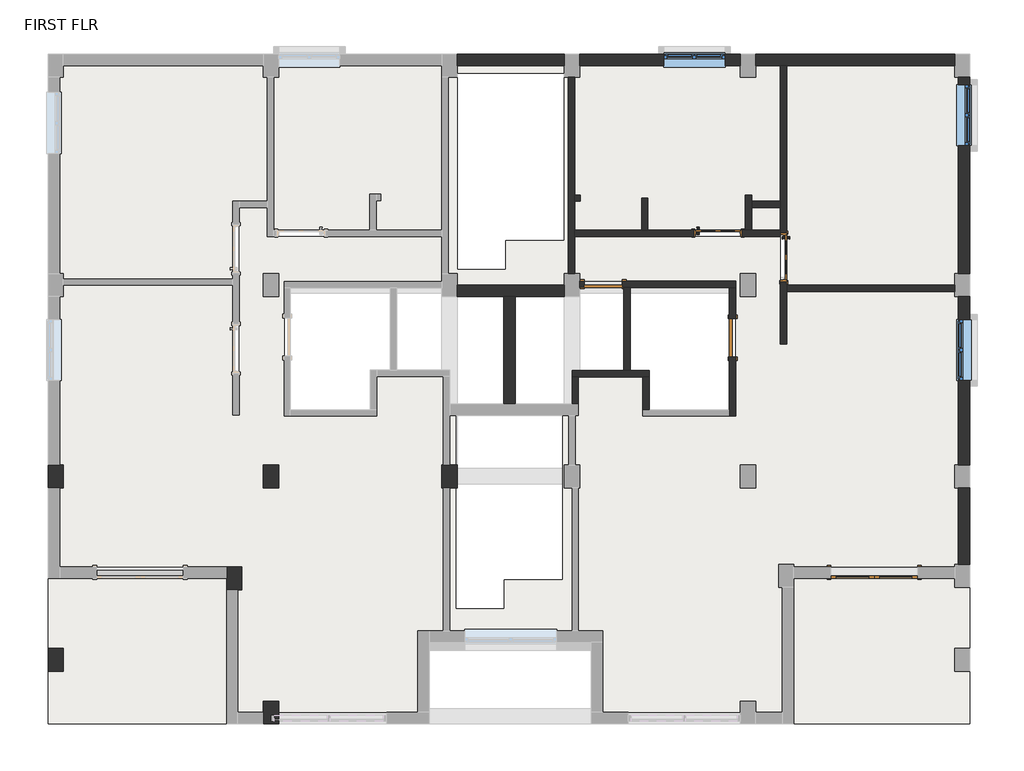
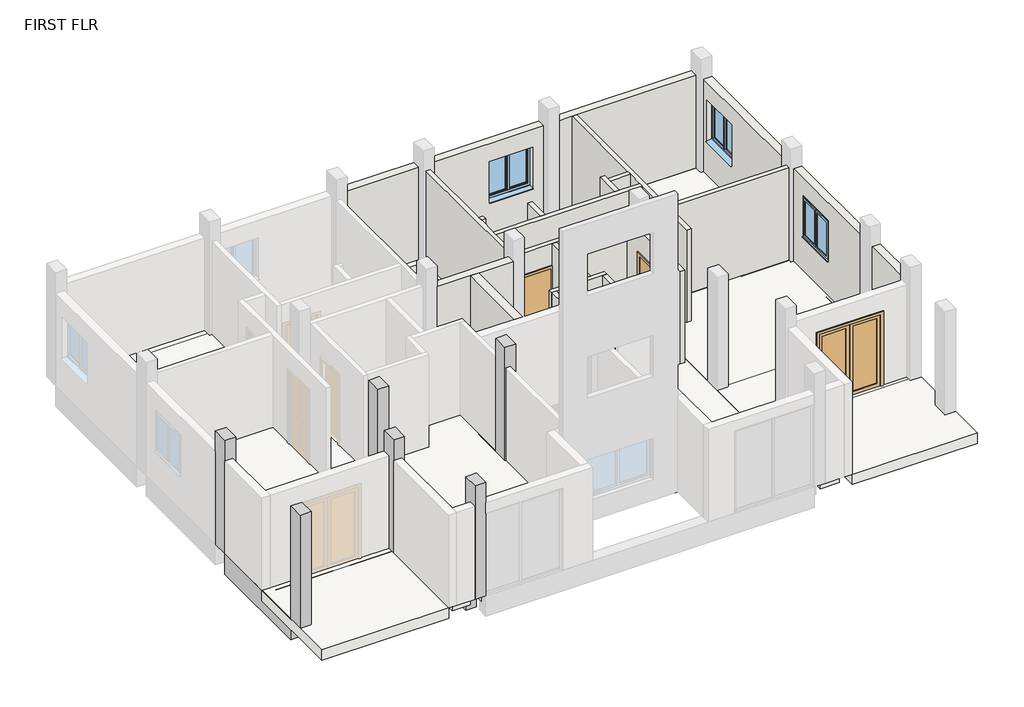
# One storey, part 2 of 3: 22 walls, 7 slabs, 6 beams, 6 columns, 5 doors, 3 windows.
"""IFC4 building model written with IfcOpenShell, lengths in millimetres."""

from ifc_helpers import new_model, si_unit, frame, origin, place, context, project, spatial, polyline, outline, extrude, faceted_brep, transform, mapped, element, save
from components import door_e52a3823, door_68a706ac, door_1fe7f57d, w2_0001_windows_4_x_4_9dec5fc7

model = new_model("IFC4")

# Units and contexts
model_context = context("Model", 3, world=origin())
ifc_project = project(units=[si_unit("LENGTHUNIT", "METRE", prefix="MILLI")], contexts=[model_context])

# Site, building, storey
site = spatial("IfcSite", under=ifc_project)
building = spatial("IfcBuilding", under=site)
storey = spatial("IfcBuildingStorey", under=building, Name="FIRST FLR", Elevation=3352.8)

# Beams
placement = place(None, origin())
element("IfcBeam", 1, ObjectType="Concrete-Rectangular Beam : 12 x 24", at=placement, inside=storey, context=model_context, shape_type="Brep", body=[
    faceted_brep([(-9144.7786397, -13068.2620333, 3352.8), (-8839.9786397, -13068.2620333, 3352.8), (-8839.9786397, -11823.6620333, 3352.8), (-8839.9786397, -11518.8620333, 3352.8), (-8839.9786397, -9867.8620333, 3352.8), (-9144.7786397, -9867.8620333, 3352.8), (-9144.7786397, -13068.2620333, 2743.2), (-9144.7786397, -9867.8620333, 2743.2), (-8839.9786397, -13068.2620333, 2743.2), (-8839.9786397, -9867.8620333, 2743.2), (-8839.9786397, -11518.8620333, 2743.2), (-8839.9786397, -11823.6620333, 2743.2)], [[[0, 1, 2, 3, 4, 5]], [[6, 0, 5, 7]], [[8, 6, 7, 9, 10, 11]], [[1, 8, 11, 10, 9, 4, 3, 2]], [[4, 9, 7, 5]], [[1, 0, 6, 8]]]),
])
element("IfcBeam", 2, ObjectType="Concrete-Rectangular Beam : 12 x 24", at=placement, inside=storey, context=model_context, shape_type="SweptSolid", body=[
    extrude(outline(polyline([(-4852.9175798, -9486.8620333), (-4852.9175798, -9791.6620333), (-8839.9786397, -9791.6620333), (-8839.9786397, -9486.8620333), (-4852.9175798, -9486.8620333)])), frame((0.0, 0.0, 2743.2), z_axis=(0.0, 0.0, 1.0), x_axis=(1.0, 0.0, 0.0)), (0.0, 0.0, 1.0), 609.6),
])
element("IfcBeam", 3, ObjectType="Concrete-Rectangular Beam : 12 x 24", at=placement, inside=storey, context=model_context, shape_type="SweptSolid", body=[
    extrude(outline(polyline([(-1296.9175798, -9486.8620333), (-1296.9175798, -9791.6620333), (-4548.1175798, -9791.6620333), (-4548.1175798, -9486.8620333), (-1296.9175798, -9486.8620333)])), frame((0.0, 0.0, 2743.2), z_axis=(0.0, 0.0, 1.0), x_axis=(1.0, 0.0, 0.0)), (0.0, 0.0, 1.0), 609.6),
])
element("IfcBeam", 4, ObjectType="Concrete-Rectangular Beam : 12 x 24", at=placement, inside=storey, context=model_context, shape_type="Brep", body=[
    faceted_brep([(-4852.9175798, -14119.6402089, 3352.8), (-4548.1175798, -14119.6402089, 3352.8), (-4548.1175798, -9867.8620333, 3352.8), (-4852.9175798, -9867.8620333, 3352.8), (-4852.9175798, -11518.8620333, 3352.8), (-4852.9175798, -11823.6620333, 3352.8), (-4852.9175798, -14119.6402089, 2743.2), (-4852.9175798, -9867.8620333, 2743.2), (-4852.9175798, -11518.8620333, 2743.2), (-4852.9175798, -11823.6620333, 2743.2), (-4548.1175798, -14119.6402089, 2743.2), (-4548.1175798, -9867.8620333, 2743.2)], [[[0, 1, 2, 3, 4, 5]], [[6, 0, 5, 4, 3, 7, 8, 9]], [[10, 6, 9, 8, 7, 11]], [[1, 10, 11, 2]], [[2, 11, 7, 3]], [[1, 0, 6, 10]]]),
])
element("IfcBeam", 5, ObjectType="Concrete-Rectangular Beam : 12 x 24", at=placement, inside=storey, context=model_context, shape_type="SweptSolid", body=[
    extrude(outline(polyline([(-5284.7175798, -11823.6620333), (-5284.7175798, -11518.8620333), (-4852.9175798, -11518.8620333), (-4852.9175798, -11823.6620333), (-5284.7175798, -11823.6620333)])), frame((0.0, 0.0, 2743.2), z_axis=(0.0, 0.0, 1.0), x_axis=(1.0, 0.0, 0.0)), (0.0, 0.0, 1.0), 609.6),
])
element("IfcBeam", 6, ObjectType="Concrete-Rectangular Beam : 12 x 24", at=placement, inside=storey, context=model_context, shape_type="SweptSolid", body=[
    extrude(outline(polyline([(-5589.5175798, -11518.8620333), (-5589.5175798, -11823.6620333), (-8839.9786397, -11823.6620333), (-8839.9786397, -11518.8620333), (-5589.5175798, -11518.8620333)])), frame((0.0, 0.0, 2743.2), z_axis=(0.0, 0.0, 1.0), x_axis=(1.0, 0.0, 0.0)), (0.0, 0.0, 1.0), 609.6),
])

# Columns
element("IfcColumn", 7, ObjectType="Concrete-Rectangular-Column : 1'6\" X 1' COLUMN", at=placement, inside=storey, context=model_context, shape_type="Brep", body=[
    faceted_brep([(-8839.9786397, -9410.6620333, 3352.8), (-8839.9786397, -9867.8620333, 3352.8), (-9144.7786397, -9867.8620333, 3352.8), (-9144.7786397, -9410.6620333, 3352.8), (-8839.9786397, -9410.6620333, 6705.6), (-8839.9786397, -9486.8620333, 6705.6), (-8839.9786397, -9791.6620333, 6705.6), (-8839.9786397, -9867.8620333, 6705.6), (-8839.9786397, -9867.8620333, 6096.0), (-8839.9786397, -9867.8620333, 5791.2), (-8839.9786397, -9410.6620333, 5791.2), (-8839.9786397, -9410.6620333, 6096.0), (-9144.7786397, -9867.8620333, 6705.6), (-9144.7786397, -9867.8620333, 6096.0), (-9144.7786397, -9867.8620333, 5791.2), (-9144.7786397, -9410.6620333, 6705.6), (-9144.7786397, -9410.6620333, 6096.0), (-9144.7786397, -9410.6620333, 5791.2)], [[[0, 1, 2, 3]], [[4, 5, 6, 7, 8, 9, 1, 0, 10, 11]], [[7, 12, 13, 14, 2, 1, 9, 8]], [[12, 15, 16, 17, 3, 2, 14, 13]], [[15, 4, 11, 10, 0, 3, 17, 16]], [[4, 15, 12, 7, 6, 5]]]),
])
element("IfcColumn", 8, ObjectType="Concrete-Rectangular-Column : 1'6\" X 1' COLUMN", at=placement, inside=storey, context=model_context, shape_type="Brep", body=[
    faceted_brep([(-4548.1175798, -9410.6620333, 3352.8), (-4548.1175798, -9867.8620333, 3352.8), (-4852.9175798, -9867.8620333, 3352.8), (-4852.9175798, -9410.6620333, 3352.8), (-4548.1175798, -9410.6620333, 6705.6), (-4548.1175798, -9486.8620333, 6705.6), (-4548.1175798, -9791.6620333, 6705.6), (-4548.1175798, -9867.8620333, 6705.6), (-4548.1175798, -9867.8620333, 6096.0), (-4548.1175798, -9867.8620333, 5791.2), (-4548.1175798, -9410.6620333, 5791.2), (-4548.1175798, -9410.6620333, 6096.0), (-4852.9175798, -9867.8620333, 6705.6), (-4852.9175798, -9867.8620333, 6096.0), (-4852.9175798, -9867.8620333, 5791.2), (-4852.9175798, -9791.6620333, 6705.6), (-4852.9175798, -9486.8620333, 6705.6), (-4852.9175798, -9410.6620333, 6705.6), (-4852.9175798, -9410.6620333, 6096.0), (-4852.9175798, -9410.6620333, 5791.2)], [[[0, 1, 2, 3]], [[4, 5, 6, 7, 8, 9, 1, 0, 10, 11]], [[7, 12, 13, 14, 2, 1, 9, 8]], [[12, 15, 16, 17, 18, 19, 3, 2, 14, 13]], [[17, 4, 11, 10, 0, 3, 19, 18]], [[4, 17, 16, 15, 12, 7, 6, 5]]]),
])
element("IfcColumn", 9, ObjectType="Concrete-Rectangular-Column : 1'6\" X 1' COLUMN", at=placement, inside=storey, context=model_context, shape_type="Brep", body=[
    faceted_brep([(-992.1175798, -9410.6620333, 3352.8), (-992.1175798, -9867.8620333, 3352.8), (-1296.9175798, -9867.8620333, 3352.8), (-1296.9175798, -9410.6620333, 3352.8), (-992.1175798, -9410.6620333, 6705.6), (-992.1175798, -9867.8620333, 6705.6), (-992.1175798, -9410.6620333, 5791.2), (-992.1175798, -9410.6620333, 6096.0), (-1296.9175798, -9867.8620333, 6705.6), (-1296.9175798, -9791.6620333, 6705.6), (-1296.9175798, -9486.8620333, 6705.6), (-1296.9175798, -9410.6620333, 6705.6), (-1296.9175798, -9410.6620333, 6096.0), (-1296.9175798, -9410.6620333, 5791.2)], [[[0, 1, 2, 3]], [[4, 5, 1, 0, 6, 7]], [[5, 8, 2, 1]], [[8, 9, 10, 11, 12, 13, 3, 2]], [[11, 4, 7, 6, 0, 3, 13, 12]], [[4, 11, 10, 9, 8, 5]]]),
])
element("IfcColumn", 10, ObjectType="Concrete-Rectangular-Column : 1'6\" X 1' COLUMN", at=placement, inside=storey, context=model_context, shape_type="Brep", body=[
    faceted_brep([(-4548.1175798, -14119.6402089, 3352.8), (-4548.1175798, -14576.8402089, 3352.8), (-4852.9175798, -14576.8402089, 3352.8), (-4852.9175798, -14119.6402089, 3352.8), (-4548.1175798, -14119.6402089, 6705.6), (-4548.1175798, -14576.8402089, 6705.6), (-4548.1175798, -14576.8402089, 6400.8), (-4548.1175798, -14576.8402089, 5791.2), (-4548.1175798, -14119.6402089, 5791.2), (-4548.1175798, -14119.6402089, 6096.0), (-4852.9175798, -14576.8402089, 6705.6), (-4852.9175798, -14119.6402089, 6705.6), (-4852.9175798, -14119.6402089, 6096.0), (-4852.9175798, -14119.6402089, 5791.2)], [[[0, 1, 2, 3]], [[4, 5, 6, 7, 1, 0, 8, 9]], [[5, 10, 2, 1, 7, 6]], [[10, 11, 12, 13, 3, 2]], [[11, 4, 9, 8, 0, 3, 13, 12]], [[4, 11, 10, 5]]]),
])
element("IfcColumn", 11, ObjectType="Concrete-Rectangular-Column : 1'6\" X 1' COLUMN", at=placement, inside=storey, context=model_context, shape_type="Brep", body=[
    faceted_brep([(-8839.9786397, -13068.2620333, 3352.8), (-8839.9786397, -13525.4620333, 3352.8), (-9144.7786397, -13525.4620333, 3352.8), (-9144.7786397, -13068.2620333, 3352.8), (-8839.9786397, -13068.2620333, 6705.6), (-8839.9786397, -13525.4620333, 6705.6), (-8839.9786397, -13068.2620333, 5791.2), (-8839.9786397, -13068.2620333, 6096.0), (-9144.7786397, -13525.4620333, 6705.6), (-9144.7786397, -13068.2620333, 6705.6), (-9144.7786397, -13068.2620333, 6096.0), (-9144.7786397, -13068.2620333, 5791.2)], [[[0, 1, 2, 3]], [[4, 5, 1, 0, 6, 7]], [[5, 8, 2, 1]], [[8, 9, 10, 11, 3, 2]], [[9, 4, 7, 6, 0, 3, 11, 10]], [[4, 9, 8, 5]]]),
])
element("IfcColumn", 12, ObjectType="Concrete-Rectangular-Column : 1'6\" X 1' COLUMN", at=placement, inside=storey, context=model_context, shape_type="SweptSolid", body=[
    extrude(outline(polyline([(-5284.7175798, -11442.6620333), (-5284.7175798, -11899.8620333), (-5589.5175798, -11899.8620333), (-5589.5175798, -11442.6620333), (-5284.7175798, -11442.6620333)])), frame((0.0, 0.0, 3352.8), z_axis=(0.0, 0.0, 1.0), x_axis=(1.0, 0.0, 0.0)), (0.0, 0.0, 1.0), 3352.8),
])

# Doors
door_shape = door_e52a3823(model_context)
element("IfcDoor", 13, ObjectType="Door-Double-Glass : 68\" x 84\"", at=placement, inside=storey, context=model_context, shape_type="MappedRepresentation", body=[
    mapped(door_shape, transform((7313.6824202, -11554.5807833, 3352.8), x_axis=(-1.0, 0.0, 0.0), y_axis=(0.0, -1.0, 0.0), z_axis=(0.0, 0.0, 1.0))),
])
door_2_shape = door_68a706ac(model_context)
element("IfcDoor", 14, ObjectType="Door-Interior-Single-4_Panel-Wood : 36\" x 84\"", at=placement, inside=storey, context=model_context, shape_type="MappedRepresentation", body=[
    mapped(door_2_shape, transform((4202.1824202, -4789.1311634, 3352.8), x_axis=(1.0, 0.0, 0.0), y_axis=(0.0, 1.0, 0.0), z_axis=(0.0, 0.0, 1.0))),
])
element("IfcDoor", 15, ObjectType="Door-Interior-Single-4_Panel-Wood : 36\" x 84\"", at=placement, inside=storey, context=model_context, shape_type="MappedRepresentation", body=[
    mapped(door_2_shape, transform((5513.4574202, -5274.9061634, 3352.8), x_axis=(0.0, -1.0, 0.0), y_axis=(1.0, 0.0, 0.0), z_axis=(0.0, 0.0, 1.0))),
])
door_3_shape = door_1fe7f57d(model_context)
element("IfcDoor", 16, ObjectType="Single-Flush : 30\" x 80\"", at=placement, inside=storey, context=model_context, shape_type="MappedRepresentation", body=[
    mapped(door_3_shape, transform((1916.1824202, -5810.8691591, 3352.8), x_axis=(-1.0, 0.0, 0.0), y_axis=(0.0, -1.0, 0.0), z_axis=(0.0, 0.0, 1.0))),
])
element("IfcDoor", 17, ObjectType="Single-Flush : 30\" x 80\"", at=placement, inside=storey, context=model_context, shape_type="MappedRepresentation", body=[
    mapped(door_3_shape, transform((4494.2824202, -6877.6691591, 3352.8), x_axis=(0.0, 1.0, 0.0), y_axis=(-1.0, 0.0, 0.0), z_axis=(0.0, 0.0, 1.0))),
])

# Slabs
element("IfcSlab", 18, ObjectType="flooring 1'", at=placement, inside=storey, context=model_context, shape_type="SweptSolid", body=[
    extrude(outline(polyline([(-8916.1786397, -11442.6620333), (-8916.1786397, -9867.8620333), (-8839.9786397, -9867.8620333), (-8839.9786397, -9410.6620333), (-8916.1786397, -9410.6620333), (-8916.1786397, -6057.8620333), (-8839.9786397, -6057.8620333), (-8839.9786397, -5829.2620333), (-5462.5175798, -5829.2620333), (-5462.5175798, -8420.0620333), (-5335.5175798, -8420.0620333), (-5335.5175798, -4280.3104011), (-4776.7175798, -4280.3104011), (-4776.7175798, -4855.8061634), (-1296.9175798, -4855.8061634), (-1296.9175798, -5600.6620333), (-1296.9175798, -5758.8942903), (-4442.5950401, -5758.8942903), (-4442.5950401, -8439.1120333), (-2601.0950401, -8439.1120333), (-2601.0950401, -7651.7120333), (-1271.5175798, -7651.7120333), (-1271.5175798, -9410.6620333), (-1296.9175798, -9410.6620333), (-1296.9175798, -9867.8620333), (-1271.5175798, -9867.8620333), (-1271.5175798, -12722.6402089), (-1779.5175798, -12722.6402089), (-1779.5175798, -14348.2402089), (-4548.1175798, -14348.2402089), (-4548.1175798, -14119.6402089), (-4852.9175798, -14119.6402089), (-4852.9175798, -14348.2402089), (-5360.9175798, -14348.2402089), (-5360.9175798, -11899.8620333), (-5284.7175798, -11899.8620333), (-5284.7175798, -11442.6620333), (-5589.5175798, -11442.6620333), (-8916.1786397, -11442.6620333)])), frame((0.0, 0.0, 3048.0), z_axis=(0.0, 0.0, 1.0), x_axis=(1.0, 0.0, 0.0)), (0.0, 0.0, 1.0), 304.8),
])
element("IfcSlab", 19, ObjectType="flooring 1'", at=placement, inside=storey, context=model_context, shape_type="SweptSolid", body=[
    extrude(outline(polyline([(5446.7824202, -4855.8061634), (5446.7824202, -6583.0061634), (5573.7824202, -6583.0061634), (5573.7824202, -5956.2620333), (8913.8824202, -5956.2620333), (8913.8824202, -6057.8620333), (8990.0824202, -6057.8620333), (8990.0824202, -9410.6620333), (8913.8824202, -9410.6620333), (8913.8824202, -9867.8620333), (8990.0824202, -9867.8620333), (8990.0824202, -11391.8620333), (8913.8824202, -11391.8620333), (8913.8824202, -11442.6620333), (5713.4824202, -11442.6620333), (5713.4824202, -11391.8620333), (5408.6824202, -11391.8620333), (5408.6824202, -11849.0620333), (5484.8824202, -11849.0620333), (5484.8824202, -14348.2402089), (4951.4824202, -14348.2402089), (4951.4824202, -14119.6402089), (4646.6824202, -14119.6402089), (4646.6824202, -14348.2402089), (1903.4824202, -14348.2402089), (1903.4824202, -12722.6402089), (1420.8824202, -12722.6402089), (1420.8824202, -9867.8620333), (1446.2824202, -9867.8620333), (1446.2824202, -9410.6620333), (1357.3824202, -9410.6620333), (1357.3824202, -8426.4120333), (1420.8824202, -8426.4120333), (1420.8824202, -7660.8890971), (2703.5824202, -7660.8890971), (2703.5824202, -8439.7691591), (4557.7824202, -8439.7691591), (4557.7824202, -5747.3691591), (1446.2824202, -5747.3691591), (1446.2824202, -5600.6620333), (1344.6824202, -5600.6620333), (1344.6824202, -4855.8061634), (5446.7824202, -4855.8061634)])), frame((0.0, 0.0, 3048.0), z_axis=(0.0, 0.0, 1.0), x_axis=(1.0, 0.0, 0.0)), (0.0, 0.0, 1.0), 304.8),
])
element("IfcSlab", 20, ObjectType="flooring 1'", at=placement, inside=storey, context=model_context, shape_type="SweptSolid", body=[
    extrude(outline(polyline([(-8839.9786397, -1680.8061634), (-8839.9786397, -1452.2061634), (-4852.9175798, -1452.2061634), (-4852.9175798, -1680.8061634), (-4776.7175798, -1680.8061634), (-4776.7175798, -4153.3104011), (-5462.5175798, -4153.3104011), (-5462.5175798, -5702.2620333), (-8839.9786397, -5702.2620333), (-8839.9786397, -5600.6620333), (-8916.1786397, -5600.6620333), (-8916.1786397, -1680.8061634), (-8839.9786397, -1680.8061634)])), frame((0.0, 0.0, 3048.0), z_axis=(0.0, 0.0, 1.0), x_axis=(1.0, 0.0, 0.0)), (0.0, 0.0, 1.0), 304.8),
    extrude(outline(polyline([(-2732.0175798, -4728.8061634), (-4649.7175798, -4728.8061634), (-4649.7175798, -1680.8061634), (-4548.1175798, -1680.8061634), (-4548.1175798, -1452.2061634), (-1296.9175798, -1452.2061634), (-1296.9175798, -4728.8061634), (-2605.0175798, -4728.8061634), (-2605.0175798, -4144.6061634), (-2516.1175798, -4144.6061634), (-2516.1175798, -4017.6061634), (-2732.0175798, -4017.6061634), (-2732.0175798, -4728.8061634)])), frame((0.0, 0.0, 3048.0), z_axis=(0.0, 0.0, 1.0), x_axis=(1.0, 0.0, 0.0)), (0.0, 0.0, 1.0), 304.8),
])
element("IfcSlab", 21, ObjectType="flooring 1'", at=placement, inside=storey, context=model_context, shape_type="SweptSolid", body=[
    extrude(outline(polyline([(4646.6824202, -1452.2061634), (4646.6824202, -1680.8061634), (4951.4824202, -1680.8061634), (4951.4824202, -1452.2061634), (5446.7824202, -1452.2061634), (5446.7824202, -4157.3061634), (4875.2824202, -4157.3061634), (4875.2824202, -4030.3061634), (4748.2824202, -4030.3061634), (4748.2824202, -4728.8061634), (2805.1824202, -4728.8061634), (2805.1824202, -4093.8061634), (2678.1824202, -4093.8061634), (2678.1824202, -4728.8061634), (1344.6824202, -4728.8061634), (1344.6824202, -4157.3061634), (1458.9824202, -4157.3061634), (1458.9824202, -4030.3061634), (1344.6824202, -4030.3061634), (1344.6824202, -1680.8061634), (1446.2824202, -1680.8061634), (1446.2824202, -1452.2061634), (4646.6824202, -1452.2061634)])), frame((0.0, 0.0, 3048.0), z_axis=(0.0, 0.0, 1.0), x_axis=(1.0, 0.0, 0.0)), (0.0, 0.0, 1.0), 304.8),
    extrude(outline(polyline([(5446.7824202, -4284.3061634), (5446.7824202, -4728.8061634), (4875.2824202, -4728.8061634), (4875.2824202, -4284.3061634), (5446.7824202, -4284.3061634)])), frame((0.0, 0.0, 3048.0), z_axis=(0.0, 0.0, 1.0), x_axis=(1.0, 0.0, 0.0)), (0.0, 0.0, 1.0), 304.8),
    extrude(outline(polyline([(8913.8824202, -5829.2620333), (5573.7824202, -5829.2620333), (5573.7824202, -1452.2061634), (8913.8824202, -1452.2061634), (8913.8824202, -1680.8061634), (8990.0824202, -1680.8061634), (8990.0824202, -5600.6620333), (8913.8824202, -5600.6620333), (8913.8824202, -5829.2620333)])), frame((0.0, 0.0, 3048.0), z_axis=(0.0, 0.0, 1.0), x_axis=(1.0, 0.0, 0.0)), (0.0, 0.0, 1.0), 304.8),
])
element("IfcSlab", 22, ObjectType="flooring 1'", at=placement, inside=storey, context=model_context, shape_type="SweptSolid", body=[
    extrude(outline(polyline([(1141.4824202, -1680.8061634), (1217.6824202, -1680.8061634), (1217.6824202, -5600.6620333), (1141.4824202, -5600.6620333), (1141.4824202, -5829.2620333), (-992.1175798, -5829.2620333), (-992.1175798, -5600.6620333), (-1169.9175798, -5600.6620333), (-1169.9175798, -1680.8061634), (-992.1175798, -1680.8061634), (-992.1175798, -5516.2061634), (-26.9175798, -5516.2061634), (-26.9175798, -4938.3561634), (1141.4824202, -4938.3561634), (1141.4824202, -1680.8061634)])), frame((0.0, 0.0, 3048.0), z_axis=(0.0, 0.0, 1.0), x_axis=(1.0, 0.0, 0.0)), (0.0, 0.0, 1.0), 304.8),
    extrude(outline(polyline([(-992.1175798, -1452.2061634), (1141.4824202, -1452.2061634), (1141.4824202, -1604.6061634), (-992.1175798, -1604.6061634), (-992.1175798, -1452.2061634)])), frame((0.0, 0.0, 3048.0), z_axis=(0.0, 0.0, 1.0), x_axis=(1.0, 0.0, 0.0)), (0.0, 0.0, 1.0), 304.8),
])
element("IfcSlab", 23, ObjectType="flooring 1'", at=placement, inside=storey, context=model_context, shape_type="SweptSolid", body=[
    extrude(outline(polyline([(1293.8824202, -12722.6402089), (-1144.5175798, -12722.6402089), (-1144.5175798, -9867.8620333), (-1023.6148833, -9867.8620333), (-1023.6148833, -12279.1584166), (-58.4148833, -12279.1584166), (-58.4148833, -11701.3084166), (1109.9851167, -11701.3084166), (1109.9851167, -8426.4120333), (1230.3824202, -8426.4120333), (1230.3824202, -9410.6620333), (1141.4824202, -9410.6620333), (1141.4824202, -9867.8620333), (1293.8824202, -9867.8620333), (1293.8824202, -12722.6402089)])), frame((0.0, 0.0, 3048.0), z_axis=(0.0, 0.0, 1.0), x_axis=(1.0, 0.0, 0.0)), (0.0, 0.0, 1.0), 304.8),
    extrude(outline(polyline([(-1144.5175798, -9410.6620333), (-1144.5175798, -8426.4120333), (-1023.6148833, -8426.4120333), (-1023.6148833, -9410.6620333), (-1144.5175798, -9410.6620333)])), frame((0.0, 0.0, 3048.0), z_axis=(0.0, 0.0, 1.0), x_axis=(1.0, 0.0, 0.0)), (0.0, 0.0, 1.0), 304.8),
])
element("IfcSlab", 24, ObjectType="flooring 1'", at=placement, inside=storey, context=model_context, shape_type="SweptSolid", body=[
    extrude(outline(polyline([(-5589.5175798, -11671.2620333), (-5589.5175798, -14576.8402089), (-9144.7786397, -14576.8402089), (-9144.7786397, -11671.2620333), (-5589.5175798, -11671.2620333)])), frame((0.0, 0.0, 3048.0), z_axis=(0.0, 0.0, 1.0), x_axis=(1.0, 0.0, 0.0)), (0.0, 0.0, 1.0), 304.8),
    extrude(outline(polyline([(9218.6824202, -11671.2620333), (9218.6824202, -14576.8402089), (5713.4824202, -14576.8402089), (5713.4824202, -11671.2620333), (9218.6824202, -11671.2620333)])), frame((0.0, 0.0, 3048.0), z_axis=(0.0, 0.0, 1.0), x_axis=(1.0, 0.0, 0.0)), (0.0, 0.0, 1.0), 304.8),
])

# Walls
element("IfcWall", 25, ObjectType="EXTERIOR WALL 9\"", at=placement, inside=storey, context=model_context, shape_type="SweptSolid", body=[
    extrude(outline(polyline([(1141.4824202, -1452.2061634), (-992.1175798, -1452.2061634), (-992.1175798, -1223.6061634), (1141.4824202, -1223.6061634), (1141.4824202, -1452.2061634)])), frame((0.0, 0.0, 3352.8), z_axis=(0.0, 0.0, 1.0), x_axis=(1.0, 0.0, 0.0)), (0.0, 0.0, 1.0), 2743.2),
])
element("IfcWall", 26, ObjectType="EXTERIOR WALL 9\"", at=placement, inside=storey, context=model_context, shape_type="SweptSolid", body=[
    extrude(outline(polyline([(3352.8, 1446.2824202), (3352.8, 4646.6824202), (6096.0, 4646.6824202), (6096.0, 1446.2824202), (3352.8, 1446.2824202)]), holes=[polyline([(4352.8, 4341.8824202), (4352.8, 3122.6824202), (5572.0, 3122.6824202), (5572.0, 4341.8824202), (4352.8, 4341.8824202)])]), frame((0.0, -1452.2061634, 0.0), z_axis=(0.0, 1.0, 0.0), x_axis=(0.0, 0.0, 1.0)), (0.0, 0.0, 1.0), 228.6),
])
element("IfcWall", 27, ObjectType="EXTERIOR WALL 9\"", at=placement, inside=storey, context=model_context, shape_type="Brep", body=[
    faceted_brep([(4951.4824202, -1452.2061634, 3352.8), (5446.7824202, -1452.2061634, 3352.8), (5573.7824202, -1452.2061634, 3352.8), (8913.8824202, -1452.2061634, 3352.8), (8913.8824202, -1452.2061634, 6096.0), (5573.7824202, -1452.2061634, 6096.0), (5446.7824202, -1452.2061634, 6096.0), (4951.4824202, -1452.2061634, 6096.0), (4951.4824202, -1223.6061634, 3352.8), (4951.4824202, -1223.6061634, 6096.0), (8913.8824202, -1223.6061634, 6096.0), (8913.8824202, -1223.6061634, 3352.8)], [[[0, 1, 2, 3, 4, 5, 6, 7]], [[8, 9, 10, 11]], [[3, 2, 1, 0, 8, 11]], [[4, 3, 11, 10]], [[7, 6, 5, 4, 10, 9]], [[0, 7, 9, 8]]]),
])
element("IfcWall", 28, ObjectType="EXTERIOR WALL 9\"", at=placement, inside=storey, context=model_context, shape_type="SweptSolid", body=[
    extrude(outline(polyline([(-1680.8061634, 3352.8), (-5600.6620333, 3352.8), (-5600.6620333, 6096.0), (-1680.8061634, 6096.0), (-1680.8061634, 3352.8)]), holes=[polyline([(-3052.4061634, 4352.8), (-1833.2061634, 4352.8), (-1833.2061634, 5572.0), (-3052.4061634, 5572.0), (-3052.4061634, 4352.8)])]), frame((8990.0824202, 0.0, 0.0), z_axis=(1.0, 0.0, 0.0), x_axis=(0.0, 1.0, 0.0)), (0.0, 0.0, 1.0), 228.6),
])
element("IfcWall", 29, ObjectType="EXTERIOR WALL 9\"", at=placement, inside=storey, context=model_context, shape_type="SweptSolid", body=[
    extrude(outline(polyline([(-6057.8620333, 3352.8), (-9410.6620333, 3352.8), (-9410.6620333, 6096.0), (-6057.8620333, 6096.0), (-6057.8620333, 3352.8)]), holes=[polyline([(-6515.0620333, 4352.8), (-6515.0620333, 5572.0), (-7734.2620333, 5572.0), (-7734.2620333, 4352.8), (-6515.0620333, 4352.8)])]), frame((8990.0824202, 0.0, 0.0), z_axis=(1.0, 0.0, 0.0), x_axis=(0.0, 1.0, 0.0)), (0.0, 0.0, 1.0), 228.6),
])
element("IfcWall", 30, ObjectType="EXTERIOR WALL 9\"", at=placement, inside=storey, context=model_context, shape_type="SweptSolid", body=[
    extrude(outline(polyline([(8990.0824202, -11391.8620333), (8990.0824202, -9867.8620333), (9218.6824202, -9867.8620333), (9218.6824202, -11391.8620333), (8990.0824202, -11391.8620333)])), frame((0.0, 0.0, 3352.8), z_axis=(0.0, 0.0, 1.0), x_axis=(1.0, 0.0, 0.0)), (0.0, 0.0, 1.0), 2743.2),
])
element("IfcWall", 31, ObjectType="EXTERIOR WALL 9\"", at=placement, inside=storey, context=model_context, shape_type="Brep", body=[
    faceted_brep([(1141.4824202, -5829.2620333, 3352.8), (-992.1175798, -5829.2620333, 3352.8), (-992.1175798, -5829.2620333, 6096.0), (1141.4824202, -5829.2620333, 6096.0), (1141.4824202, -6057.8620333, 3352.8), (1141.4824202, -6057.8620333, 6096.0), (163.5824202, -6057.8620333, 6096.0), (-65.0175798, -6057.8620333, 6096.0), (-992.1175798, -6057.8620333, 6096.0), (-992.1175798, -6057.8620333, 3352.8), (-65.0175798, -6057.8620333, 3352.8), (163.5824202, -6057.8620333, 3352.8)], [[[0, 1, 2, 3]], [[4, 5, 6, 7, 8, 9, 10, 11]], [[1, 0, 4, 11, 10, 9]], [[2, 1, 9, 8]], [[3, 2, 8, 7, 6, 5]], [[0, 3, 5, 4]]]),
])
element("IfcWall", 32, ObjectType="EXTERIOR WALL 9\"", at=placement, inside=storey, context=model_context, shape_type="SweptSolid", body=[
    extrude(outline(polyline([(-65.0175798, -8197.8120333), (-65.0175798, -6057.8620333), (163.5824202, -6057.8620333), (163.5824202, -8197.8120333), (-65.0175798, -8197.8120333)])), frame((0.0, 0.0, 3352.8), z_axis=(0.0, 0.0, 1.0), x_axis=(1.0, 0.0, 0.0)), (0.0, 0.0, 1.0), 2743.2),
])
element("IfcWall", 33, ObjectType="INTERIOR WALL 5\"", at=placement, inside=storey, context=model_context, shape_type="Brep", body=[
    faceted_brep([(1217.6824202, -1680.8061634, 3352.8), (1217.6824202, -5600.6620333, 3352.8), (1217.6824202, -5600.6620333, 6096.0), (1217.6824202, -1680.8061634, 6096.0), (1344.6824202, -1680.8061634, 3352.8), (1344.6824202, -1680.8061634, 6096.0), (1344.6824202, -4030.3061634, 6096.0), (1344.6824202, -4157.3061634, 6096.0), (1344.6824202, -4728.8061634, 6096.0), (1344.6824202, -4855.8061634, 6096.0), (1344.6824202, -5600.6620333, 6096.0), (1344.6824202, -5600.6620333, 3352.8), (1344.6824202, -4855.8061634, 3352.8), (1344.6824202, -4728.8061634, 3352.8), (1344.6824202, -4157.3061634, 3352.8), (1344.6824202, -4030.3061634, 3352.8)], [[[0, 1, 2, 3]], [[4, 5, 6, 7, 8, 9, 10, 11, 12, 13, 14, 15]], [[1, 0, 4, 15, 14, 13, 12, 11]], [[2, 1, 11, 10]], [[3, 2, 10, 9, 8, 7, 6, 5]], [[0, 3, 5, 4]]]),
])
element("IfcWall", 34, ObjectType="INTERIOR WALL 5\"", at=placement, inside=storey, context=model_context, shape_type="Brep", body=[
    faceted_brep([(5446.7824202, -4855.8061634, 6096.0), (1344.6824202, -4855.8061634, 6096.0), (1344.6824202, -4855.8061634, 3352.8), (3719.5824202, -4855.8061634, 3352.8), (3719.5824202, -4855.8061634, 5511.8), (4684.7824202, -4855.8061634, 5511.8), (4684.7824202, -4855.8061634, 3352.8), (5446.7824202, -4855.8061634, 3352.8), (1344.6824202, -4728.8061634, 6096.0), (2678.1824202, -4728.8061634, 6096.0), (2805.1824202, -4728.8061634, 6096.0), (4748.2824202, -4728.8061634, 6096.0), (4875.2824202, -4728.8061634, 6096.0), (5446.7824202, -4728.8061634, 6096.0), (5446.7824202, -4728.8061634, 3352.8), (4875.2824202, -4728.8061634, 3352.8), (4748.2824202, -4728.8061634, 3352.8), (4684.7824202, -4728.8061634, 3352.8), (4684.7824202, -4728.8061634, 5511.8), (3719.5824202, -4728.8061634, 5511.8), (3719.5824202, -4728.8061634, 3352.8), (2805.1824202, -4728.8061634, 3352.8), (2678.1824202, -4728.8061634, 3352.8), (1344.6824202, -4728.8061634, 3352.8)], [[[0, 1, 2, 3, 4, 5, 6, 7]], [[8, 9, 10, 11, 12, 13, 14, 15, 16, 17, 18, 19, 20, 21, 22, 23]], [[2, 23, 22, 21, 20, 3]], [[14, 7, 6, 17, 16, 15]], [[1, 0, 13, 12, 11, 10, 9, 8]], [[2, 1, 8, 23]], [[0, 7, 14, 13]], [[5, 18, 17, 6]], [[18, 5, 4, 19]], [[19, 4, 3, 20]]]),
])
element("IfcWall", 35, ObjectType="INTERIOR WALL 5\"", at=placement, inside=storey, context=model_context, shape_type="Brep", body=[
    faceted_brep([(4875.2824202, -4728.8061634, 3352.8), (4875.2824202, -4284.3061634, 3352.8), (4875.2824202, -4157.3061634, 3352.8), (4875.2824202, -4030.3061634, 3352.8), (4875.2824202, -4030.3061634, 6096.0), (4875.2824202, -4157.3061634, 6096.0), (4875.2824202, -4284.3061634, 6096.0), (4875.2824202, -4728.8061634, 6096.0), (4748.2824202, -4728.8061634, 3352.8), (4748.2824202, -4728.8061634, 6096.0), (4748.2824202, -4030.3061634, 6096.0), (4748.2824202, -4030.3061634, 3352.8)], [[[0, 1, 2, 3, 4, 5, 6, 7]], [[8, 9, 10, 11]], [[3, 2, 1, 0, 8, 11]], [[4, 3, 11, 10]], [[7, 6, 5, 4, 10, 9]], [[0, 7, 9, 8]]]),
])
element("IfcWall", 36, ObjectType="INTERIOR WALL 5\"", at=placement, inside=storey, context=model_context, shape_type="SweptSolid", body=[
    extrude(outline(polyline([(5446.7824202, -4284.3061634), (4875.2824202, -4284.3061634), (4875.2824202, -4157.3061634), (5446.7824202, -4157.3061634), (5446.7824202, -4284.3061634)])), frame((0.0, 0.0, 3352.8), z_axis=(0.0, 0.0, 1.0), x_axis=(1.0, 0.0, 0.0)), (0.0, 0.0, 1.0), 2743.2),
])
element("IfcWall", 37, ObjectType="INTERIOR WALL 5\"", at=placement, inside=storey, context=model_context, shape_type="Brep", body=[
    faceted_brep([(5446.7824202, -7002.1061634, 3352.8), (5446.7824202, -7002.1061634, 6096.0), (5446.7824202, -4855.8061634, 6096.0), (5446.7824202, -4728.8061634, 6096.0), (5446.7824202, -4284.3061634, 6096.0), (5446.7824202, -4157.3061634, 6096.0), (5446.7824202, -1452.2061634, 6096.0), (5446.7824202, -1452.2061634, 3352.8), (5446.7824202, -4157.3061634, 3352.8), (5446.7824202, -4284.3061634, 3352.8), (5446.7824202, -4728.8061634, 3352.8), (5446.7824202, -4792.3061634, 3352.8), (5446.7824202, -4792.3061634, 5511.8), (5446.7824202, -5757.5061634, 5511.8), (5446.7824202, -5757.5061634, 3352.8), (5573.7824202, -7002.1061634, 6096.0), (5573.7824202, -7002.1061634, 3352.8), (5573.7824202, -5956.2620333, 3352.8), (5573.7824202, -5829.2620333, 3352.8), (5573.7824202, -5757.5061634, 3352.8), (5573.7824202, -5757.5061634, 5511.8), (5573.7824202, -4792.3061634, 5511.8), (5573.7824202, -4792.3061634, 3352.8), (5573.7824202, -1452.2061634, 3352.8), (5573.7824202, -1452.2061634, 6096.0), (5573.7824202, -5829.2620333, 6096.0), (5573.7824202, -5956.2620333, 6096.0)], [[[0, 1, 2, 3, 4, 5, 6, 7, 8, 9, 10, 11, 12, 13, 14]], [[15, 16, 17, 18, 19, 20, 21, 22, 23, 24, 25, 26]], [[16, 0, 14, 19, 18, 17]], [[7, 23, 22, 11, 10, 9, 8]], [[1, 0, 16, 15]], [[6, 5, 4, 3, 2, 1, 15, 26, 25, 24]], [[7, 6, 24, 23]], [[13, 20, 19, 14]], [[20, 13, 12, 21]], [[21, 12, 11, 22]]]),
])
element("IfcWall", 38, ObjectType="INTERIOR WALL 5\"", at=placement, inside=storey, context=model_context, shape_type="SweptSolid", body=[
    extrude(outline(polyline([(5573.7824202, -5829.2620333), (8913.8824202, -5829.2620333), (8913.8824202, -5956.2620333), (5573.7824202, -5956.2620333), (5573.7824202, -5829.2620333)])), frame((0.0, 0.0, 3352.8), z_axis=(0.0, 0.0, 1.0), x_axis=(1.0, 0.0, 0.0)), (0.0, 0.0, 1.0), 2743.2),
])
element("IfcWall", 39, ObjectType="INTERIOR WALL 5\"", at=placement, inside=storey, context=model_context, shape_type="SweptSolid", body=[
    extrude(outline(polyline([(2805.1824202, -4093.8061634), (2805.1824202, -4728.8061634), (2678.1824202, -4728.8061634), (2678.1824202, -4093.8061634), (2805.1824202, -4093.8061634)])), frame((0.0, 0.0, 3352.8), z_axis=(0.0, 0.0, 1.0), x_axis=(1.0, 0.0, 0.0)), (0.0, 0.0, 1.0), 2743.2),
])
element("IfcWall", 40, ObjectType="INTERIOR WALL 5\"", at=placement, inside=storey, context=model_context, shape_type="SweptSolid", body=[
    extrude(outline(polyline([(1458.9824202, -4157.3061634), (1344.6824202, -4157.3061634), (1344.6824202, -4030.3061634), (1458.9824202, -4030.3061634), (1458.9824202, -4157.3061634)])), frame((0.0, 0.0, 3352.8), z_axis=(0.0, 0.0, 1.0), x_axis=(1.0, 0.0, 0.0)), (0.0, 0.0, 1.0), 2743.2),
])
element("IfcWall", 41, ObjectType="INTERIOR WALL 5\"", at=placement, inside=storey, context=model_context, shape_type="Brep", body=[
    faceted_brep([(1535.1824202, -5747.3691591, 5384.8), (1535.1824202, -5747.3691591, 3352.8), (1446.2824202, -5747.3691591, 3352.8), (1446.2824202, -5747.3691591, 6096.0), (4557.7824202, -5747.3691591, 6096.0), (4557.7824202, -5747.3691591, 3352.8), (2297.1824202, -5747.3691591, 3352.8), (2297.1824202, -5747.3691591, 5384.8), (1446.2824202, -5874.3691591, 3352.8), (1535.1824202, -5874.3691591, 3352.8), (1535.1824202, -5874.3691591, 5384.8), (2297.1824202, -5874.3691591, 5384.8), (2297.1824202, -5874.3691591, 3352.8), (2322.5824202, -5874.3691591, 3352.8), (2449.5824202, -5874.3691591, 3352.8), (4430.7824202, -5874.3691591, 3352.8), (4557.7824202, -5874.3691591, 3352.8), (4557.7824202, -5874.3691591, 6096.0), (4430.7824202, -5874.3691591, 6096.0), (2449.5824202, -5874.3691591, 6096.0), (2322.5824202, -5874.3691591, 6096.0), (1446.2824202, -5874.3691591, 6096.0)], [[[0, 1, 2, 3, 4, 5, 6, 7]], [[8, 9, 10, 11, 12, 13, 14, 15, 16, 17, 18, 19, 20, 21]], [[6, 5, 16, 15, 14, 13, 12]], [[2, 1, 9, 8]], [[3, 2, 8, 21]], [[4, 3, 21, 20, 19, 18, 17]], [[5, 4, 17, 16]], [[10, 9, 1, 0]], [[11, 10, 0, 7]], [[12, 11, 7, 6]]]),
])
element("IfcWall", 42, ObjectType="INTERIOR WALL 5\"", at=placement, inside=storey, context=model_context, shape_type="Brep", body=[
    faceted_brep([(4430.7824202, -5874.3691591, 3352.8), (4430.7824202, -6496.6691591, 3352.8), (4430.7824202, -6496.6691591, 5384.8), (4430.7824202, -7258.6691591, 5384.8), (4430.7824202, -7258.6691591, 3352.8), (4430.7824202, -8312.7691591, 3352.8), (4430.7824202, -8439.7691591, 3352.8), (4430.7824202, -8439.7691591, 6096.0), (4430.7824202, -8312.7691591, 6096.0), (4430.7824202, -5874.3691591, 6096.0), (4557.7824202, -6496.6691591, 5384.8), (4557.7824202, -6496.6691591, 3352.8), (4557.7824202, -5874.3691591, 3352.8), (4557.7824202, -5874.3691591, 6096.0), (4557.7824202, -8439.7691591, 6096.0), (4557.7824202, -8439.7691591, 3352.8), (4557.7824202, -7258.6691591, 3352.8), (4557.7824202, -7258.6691591, 5384.8)], [[[0, 1, 2, 3, 4, 5, 6, 7, 8, 9]], [[10, 11, 12, 13, 14, 15, 16, 17]], [[16, 15, 6, 5, 4]], [[12, 11, 1, 0]], [[9, 8, 7, 14, 13]], [[0, 9, 13, 12]], [[7, 6, 15, 14]], [[2, 1, 11, 10]], [[3, 2, 10, 17]], [[4, 3, 17, 16]]]),
])
element("IfcWall", 43, ObjectType="INTERIOR WALL 5\"", at=placement, inside=storey, context=model_context, shape_type="SweptSolid", body=[
    extrude(outline(polyline([(2830.5824202, -7660.8890971), (2830.5824202, -8312.7691591), (2703.5824202, -8312.7691591), (2703.5824202, -7660.8890971), (2830.5824202, -7660.8890971)])), frame((0.0, 0.0, 3352.8), z_axis=(0.0, 0.0, 1.0), x_axis=(1.0, 0.0, 0.0)), (0.0, 0.0, 1.0), 2743.2),
])
element("IfcWall", 44, ObjectType="INTERIOR WALL 5\"", at=placement, inside=storey, context=model_context, shape_type="Brep", body=[
    faceted_brep([(2830.5824202, -7533.8890971, 3352.8), (2449.5824202, -7533.8890971, 3352.8), (2322.5824202, -7533.8890971, 3352.8), (1293.8824202, -7533.8890971, 3352.8), (1293.8824202, -7533.8890971, 6096.0), (2322.5824202, -7533.8890971, 6096.0), (2449.5824202, -7533.8890971, 6096.0), (2830.5824202, -7533.8890971, 6096.0), (2830.5824202, -7660.8890971, 3352.8), (2830.5824202, -7660.8890971, 6096.0), (2703.5824202, -7660.8890971, 6096.0), (1420.8824202, -7660.8890971, 6096.0), (1293.8824202, -7660.8890971, 6096.0), (1293.8824202, -7660.8890971, 3352.8), (1420.8824202, -7660.8890971, 3352.8), (2703.5824202, -7660.8890971, 3352.8)], [[[0, 1, 2, 3, 4, 5, 6, 7]], [[8, 9, 10, 11, 12, 13, 14, 15]], [[3, 2, 1, 0, 8, 15, 14, 13]], [[7, 6, 5, 4, 12, 11, 10, 9]], [[0, 7, 9, 8]], [[4, 3, 13, 12]]]),
])
element("IfcWall", 45, ObjectType="INTERIOR WALL 5\"", at=placement, inside=storey, context=model_context, shape_type="SweptSolid", body=[
    extrude(outline(polyline([(1293.8824202, -8197.8120333), (1293.8824202, -7660.8890971), (1420.8824202, -7660.8890971), (1420.8824202, -8197.8120333), (1293.8824202, -8197.8120333)])), frame((0.0, 0.0, 3352.8), z_axis=(0.0, 0.0, 1.0), x_axis=(1.0, 0.0, 0.0)), (0.0, 0.0, 1.0), 2743.2),
])
element("IfcWall", 46, ObjectType="INTERIOR WALL 5\"", at=placement, inside=storey, context=model_context, shape_type="SweptSolid", body=[
    extrude(outline(polyline([(2322.5824202, -7533.8890971), (2322.5824202, -5874.3691591), (2449.5824202, -5874.3691591), (2449.5824202, -7533.8890971), (2322.5824202, -7533.8890971)])), frame((0.0, 0.0, 3352.8), z_axis=(0.0, 0.0, 1.0), x_axis=(1.0, 0.0, 0.0)), (0.0, 0.0, 1.0), 2743.2),
])

# Windows
w2_0001_windows_4_x_4_shape = w2_0001_windows_4_x_4_9dec5fc7(model_context)
element("IfcWindow", 47, ObjectType="w2.0001 : WINDOWS 4' X 4'", at=placement, inside=storey, context=model_context, shape_type="MappedRepresentation", body=[
    mapped(w2_0001_windows_4_x_4_shape, transform((9104.3824202, -7124.6620333, 3352.8), x_axis=(0.0, -1.0, 0.0), y_axis=(1.0, 0.0, 0.0), z_axis=(0.0, 0.0, 1.0))),
])
element("IfcWindow", 48, ObjectType="w2.0001 : WINDOWS 4' X 4'", at=placement, inside=storey, context=model_context, shape_type="MappedRepresentation", body=[
    mapped(w2_0001_windows_4_x_4_shape, transform((9104.3824202, -2442.8061634, 3352.8), x_axis=(0.0, 1.0, 0.0), y_axis=(-1.0, 0.0, 0.0), z_axis=(0.0, 0.0, 1.0))),
])
element("IfcWindow", 49, ObjectType="w2.0001 : WINDOWS 4' X 4'", at=placement, inside=storey, context=model_context, shape_type="MappedRepresentation", body=[
    mapped(w2_0001_windows_4_x_4_shape, transform((3732.2824202, -1337.9061634, 3352.8), x_axis=(-1.0, 0.0, 0.0), y_axis=(0.0, -1.0, 0.0), z_axis=(0.0, 0.0, 1.0))),
])

save(model, "model.ifc")

# Revit data of these elements
# Type "Concrete-Rectangular Beam : 12 x 24"
#   Assembly Code = "B10"
#   Length [instance default] = 5' - 0"
#   b = 1' - 0"
#   h = 2' - 0"
#   Structural Material [instance default] = Concrete, Cast-in-Place gray
# Type "Concrete-Rectangular-Column : 1'6\" X 1' COLUMN"
#   Assembly Code = "B10"
#   b = 1' - 0"
#   h = 1' - 6"
#   Structural Material [instance default] = Concrete, Cast-in-Place gray
# Type "Door-Double-Glass : 68\" x 84\""
#   Type Mark = "11"
#   Construction Type Id = "opn-d45"
#   Assembly Code = "C1020"
#   Analytic Construction = "Wood frame, double glass door "
#   W = 2' - 10"
#   Thickness = 0' - 2"
#   Thermal Resistance (R) = 1.8150 (h·ft²·°F)/BTU
#   Swing Angle [instance default] = 90.00°
#   Heat Transfer Coefficient (U) = 0.5510 BTU/(h·ft²·°F)
#   Height = 7' - 0"
#   Bottom Rail = 0' - 4"
#   Top Rail = 0' - 4"
#   Stiles = 0' - 4"
#   Trim Projection = 0' - 1"
#   Trim Width = 0' - 3"
#   Width = 5' - 8"
#   Define Thermal Properties by = 1
#   Glazing = Glass
#   Panel Material = Wood - Birch - Solid Stained Light Low Gloss
#   Trim Material = Paint - Sienna
#   Visual Light Transmittance = 0
#   Solar Heat Gain Coefficient = 0
#   Function = (empty or 0)
#   Wall Closure = (empty or 0)
# Type "Door-Interior-Single-4_Panel-Wood : 36\" x 84\""
#   Type Mark = "9"
#   Assembly Code = "C1020300"
#   Analytic Construction = "Wooden"
#   Top Rail = 0' - 4 11/16"
#   Thickness = 0' - 1 3/8"
#   Thermal Resistance (R) = 2.5876 (h·ft²·°F)/BTU
#   Swing Angle [instance default] = 90.00°
#   Stiles = 0' - 4 3/4"
#   Rough Width = 3' - 2"
#   Rough Height = 7' - 1"
#   Mullion = 0' - 4 1/2"
#   Lock Rail = 0' - 7 1/2"
#   Height = 7' - 0"
#   Width = 3' - 0"
#   Heat Transfer Coefficient (U) = 0.3865 BTU/(h·ft²·°F)
#   Bottom Rail = 0' - 9 1/8"
#   Trim Material = Cherry
#   Panel Material = Cherry
#   Frame Material = Cherry
#   Door Handle Material = Aluminum
#   Visual Light Transmittance = 0
#   Solar Heat Gain Coefficient = 0
#   Wall Closure = (empty or 0)
#   Function = (empty or 0)
# Type "Single-Flush : 30\" x 80\""
#   Type Mark = "5"
#   Construction Type Id = "MDOOR"
#   Assembly Code = "C1020"
#   Analytic Construction = "Metal"
#   Thickness = 0' - 2"
#   Heat Transfer Coefficient (U) = 0.651978 BTU/(h·ft²·°F)
#   Height = 6' - 8"
#   Trim Projection Ext = 0' - 1"
#   Trim Projection Int = 0' - 1"
#   Trim Width = 0' - 3"
#   Width = 2' - 6"
#   Define Thermal Properties by = 1
#   Define Thermal Properties by = 1
#   Door Material = Door - Panel
#   Frame Material = Door - Frame
#   Visual Light Transmittance = 0
#   Solar Heat Gain Coefficient = 0
#   Function = (empty or 0)
#   Wall Closure = (empty or 0)
# Type "flooring 1'"
#   Assembly Code = "B1010"
#   Function = 0
#   Layers, outside or top first: 1' - 0" "FL_MARBLE WHITE" (function 1)
# Type "EXTERIOR WALL 9\""
#   Assembly Code = "B2010"
#   Layers, outside or top first: 0' - 9" "WARM BEIGE COLOUR" (function 1)
# Type "INTERIOR WALL 5\""
#   Assembly Code = "B2010"
#   Layers, outside or top first: 0' - 5" "WARM BEIGE COLOUR" (function 1)
# Type "w2.0001 : WINDOWS 4' X 4'"
#   Type Mark = "21"
#   Operation = "DoublePanelVertical"
#   Keynote = "16.05.01"
#   Analytic Construction = "<None>"
#   Rough Width = 4' - 0"
#   Rough Height = 4' - 0"
#   Rahmentiefe = 0' - 2.3622"
#   Rahmenhöhe unten = 0' - 3.14961"
#   Rahmehöhe oben = 0' - 3.14961"
#   Rahmenbreite = 0' - 2.3622"
#   Height = 4' - 0"
#   Flügeltiefe = 0' - 2.3622"
#   Flügelbreite = 0' - 2.3622"
#   Einbautiefe (von außen) [instance default] = 0' - 5.51181"
#   Width = 4' - 0"
#   Kippflügel [instance default] = yes
#   Drehflügel im Grundriß darstellen [instance default] = no
#   Drehflügel [instance default] = yes
#   Define Thermal Properties by = 1
#   Rahmen [instance default] = none
#   Glas [instance default] = none
#   Flügel [instance default] = none
#   Fensterbank aussen [instance default] = none
#   Fensterbank innen [instance default] = none
#   Wall Closure = (empty or 0)
# Elements 1, 2, 3, 4, 5, 6 (IfcBeam, "Concrete-Rectangular Beam : 12 x 24")
#   Structural Material = WARM BEIGE COLOUR
#   Phase Created = New Construction
#   Materials on its faces: "WARM BEIGE COLOUR"
# Elements 7, 8, 9, 10, 11, 12 (IfcColumn, "Concrete-Rectangular-Column : 1'6\" X 1' COLUMN")
#   Structural Material = WARM BEIGE COLOUR
#   Phase Created = New Construction
#   Materials on its faces: "WARM BEIGE COLOUR"
# Element 13 (IfcDoor, "Door-Double-Glass : 68\" x 84\"")
#   Phase Created = New Construction
#   Materials on its faces: "Wood - Birch - Solid Stained Light Low Gloss", "Paint - Sienna", "Glass"
# Elements 14, 15 (IfcDoor, "Door-Interior-Single-4_Panel-Wood : 36\" x 84\"")
#   Swing Angle = 90.00°
#   Phase Created = New Construction
#   Materials on its faces: "Cherry", "Aluminum"
# Elements 16, 17 (IfcDoor, "Single-Flush : 30\" x 80\"")
#   Phase Created = New Construction
#   Materials on its faces: "Door - Frame", "Door - Panel"
# Element 18 (IfcSlab, "flooring 1'")
#   built-in parameter 1001955 = 3.14159 (stored number, unit not read)
#   Height Offset From Level = 0' - 0"
#   Phase Created = New Construction
#   Materials on its faces: "FL_MARBLE WHITE"
# Elements 19, 21, 22, 23, 24 (IfcSlab, "flooring 1'")
#   Height Offset From Level = 0' - 0"
#   Phase Created = New Construction
#   Materials on its faces: "FL_MARBLE WHITE"
# Element 20 (IfcSlab, "flooring 1'")
#   built-in parameter 1001955 = -1.5708 (stored number, unit not read)
#   Height Offset From Level = 0' - 0"
#   Phase Created = New Construction
#   Materials on its faces: "FL_MARBLE WHITE"
# Elements 25, 26, 27, 28, 29, 30, 31, 32 (IfcWall, "EXTERIOR WALL 9\"")
#   Top Offset = -1' - 0"
#   Base Offset = 0' - 0"
#   wall height = 9' - 0"
#   Phase Created = New Construction
#   Base Constraint = FIRST FLR
#   Top Constraint = Level 5
#   Materials on its faces: "WARM BEIGE COLOUR"
# Elements 33, 34, 35, 36, 37, 38, 39, 40, 41, 42, 43, 44, 45, 46 (IfcWall, "INTERIOR WALL 5\"")
#   Top Offset = -1' - 0"
#   Base Offset = 0' - 0"
#   wall height = 9' - 0"
#   Phase Created = New Construction
#   Base Constraint = FIRST FLR
#   Top Constraint = Level 5
#   Materials on its faces: "WARM BEIGE COLOUR"
# Element 47 (IfcWindow, "w2.0001 : WINDOWS 4' X 4'")
#   Mark = "17"
#   Einbautiefe (von außen) = 0' - 5.51181"
#   Kippflügel = yes
#   Drehflügel im Grundriß darstellen = no
#   Drehflügel = yes
#   Rahmen = none
#   Glas = none
#   Flügel = none
#   Fensterbank innen = none
#   Fensterbank aussen = none
#   Phase Created = New Construction
#   Materials on its faces: "Fenster - Kunststoff", "Fenster - Kunststoff weiss", "Glass", "Fenster - Holz"
# Element 48 (IfcWindow, "w2.0001 : WINDOWS 4' X 4'")
#   Mark = "18"
#   Einbautiefe (von außen) = 0' - 5.51181"
#   Kippflügel = yes
#   Drehflügel im Grundriß darstellen = no
#   Drehflügel = yes
#   Rahmen = none
#   Glas = none
#   Flügel = none
#   Fensterbank innen = none
#   Fensterbank aussen = none
#   Phase Created = New Construction
#   Materials on its faces: "Fenster - Kunststoff", "Fenster - Kunststoff weiss", "Glass", "Fenster - Holz"
# Element 49 (IfcWindow, "w2.0001 : WINDOWS 4' X 4'")
#   Mark = "19"
#   Einbautiefe (von außen) = 0' - 5.51181"
#   Kippflügel = yes
#   Drehflügel im Grundriß darstellen = no
#   Drehflügel = yes
#   Rahmen = none
#   Glas = none
#   Flügel = none
#   Fensterbank innen = none
#   Fensterbank aussen = none
#   Phase Created = New Construction
#   Materials on its faces: "Fenster - Kunststoff", "Fenster - Kunststoff weiss", "Glass", "Fenster - Holz"
# Materials
#   "Concrete, Cast-in-Place gray": class "Concrete", colour RGB 192 192 192, transparency 0, Description = "Cast-in-place concrete", Cost = 0
#   "Glass": class "Glass", colour RGB 0 128 192, transparency 0.75, Description = "Soda Lime Glass", Cost = 0
#   "Wood - Birch - Solid Stained Light Low Gloss": class "Wood", colour RGB 210 159 95, transparency 0, Cost = 0
#   "Paint - Sienna": colour RGB 118 70 51, transparency 0, Cost = 0
#   "Cherry": class "Wood", colour RGB 226 177 128, transparency 0, Description = "Prunus Serotina", Cost = 0
#   "Aluminum": class "Metal", colour RGB 247 247 247, transparency 0, Description = "Aluminum 6061", Cost = 0
#   "Door - Panel": class "Wood", colour RGB 210 159 95, transparency 0, Cost = 0
#   "Door - Frame": colour RGB 118 70 51, transparency 0, Cost = 0
#   "FL_MARBLE WHITE": class "Generic", colour RGB 120 120 120, transparency 0, Cost = 0
#   "WARM BEIGE COLOUR": class "Generic", colour RGB 120 120 120, transparency 0, Cost = 0
#   "Fenster - Kunststoff": colour RGB 249 249 249, transparency 0
#   "Fenster - Kunststoff weiss": colour RGB 249 249 249, transparency 0
#   "Fenster - Holz": colour RGB 216 135 75, transparency 0
